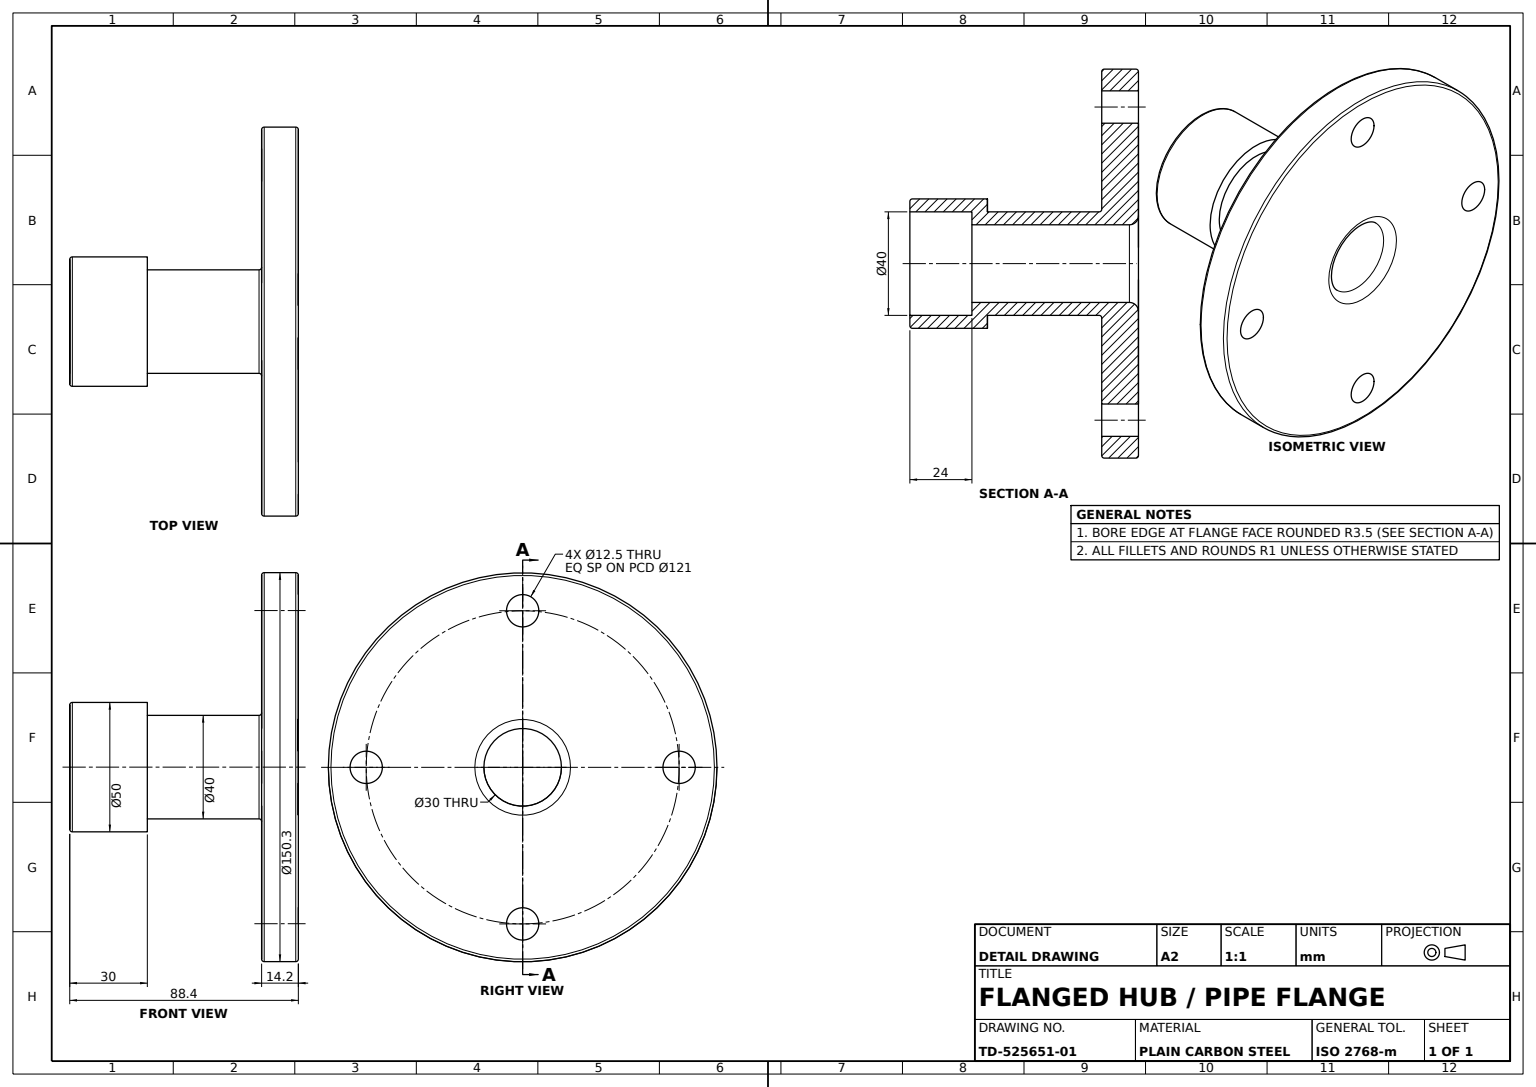
SolidWorks part; units mm, degrees
material "Plain Carbon Steel"
ref_plane "Front Plane" through (0, 0, 0) normal (0, 0, 1) x (1, 0, 0)
ref_plane "Top Plane" through (0, 0, 0) normal (0, 1, 0) x (1, 0, 0)
ref_plane "Right Plane" through (0, 0, 0) normal (1, 0, 0) x (0, 0, -1)
sketch "Connector Profile Sketch" plane through (0, 0, 0) normal (0, 0, 1) x (1, 0, 0)
  line L0 (-1000, 0) -> (49000, 0) construction
  line L2 (0, 25) -> (30, 25)
  line L3 (30, 25) -> (30, 20)
  line L4 (30, 20) -> (74.2, 20)
  line L5 (74.2, 20) -> (74.2, 75.1484)
  line L6 (74.2, 75.1484) -> (88.4, 75.1484)
  line L7 (88.4, 75.1484) -> (88.4, 15)
  line L8 (88.4, 15) -> (24, 15)
  line L9 (24, 15) -> (24, 20)
  line L10 (24, 20) -> (0, 20)
  line L11 (0, 20) -> (0, 25)
  dimension "D1" = 150.2968
  dimension "D2" = 24
  dimension "D3" = 6
  dimension "D4" = 44.2
  dimension "D5" = 14.2
  dimension "D6" = 50
  dimension "D7" = 40
  dimension "D8" = 30
  dimension "D9" = 40
revolve "Connector Body Revolve" add sketch "Connector Profile Sketch" angle 360 about L0
sketch "Bolt Holes Sketch" plane through (74.2, 0, 0) normal (-1, 0, 0) x (0, 0, 1)
  line L0 (-1000, 0) -> (49000, 0) construction
  line L1 (0, -1000) -> (0, 49000) construction
  line L2 (48.62, 0) -> (-48.62, 0) construction
  circle A0 centre (0, 60.5) radius 6.25
  circle A1 centre (0, -60.5) radius 6.25
  circle A2 centre (-60.5, 0) radius 6.25
  circle A3 centre (60.5, 0) radius 6.25
  dimension "D1" = 12.5
  dimension "D3" = 12.5
  dimension "D2" = 60.5
  dimension "D4" = 60.5
extrude "Flange Bolt Holes 4x" cut sketch "Bolt Holes Sketch" against normal blind 52
fillet "Fillet R3.5" radius 3.5 1 edges at (88.4, 0, 15)
fillet "Fillet R1" radius 1 4 edges at (88.4, 0, 75.1484) (74.2, 0, 75.1484) (74.2, 0, 20) (0, 0, 25)
